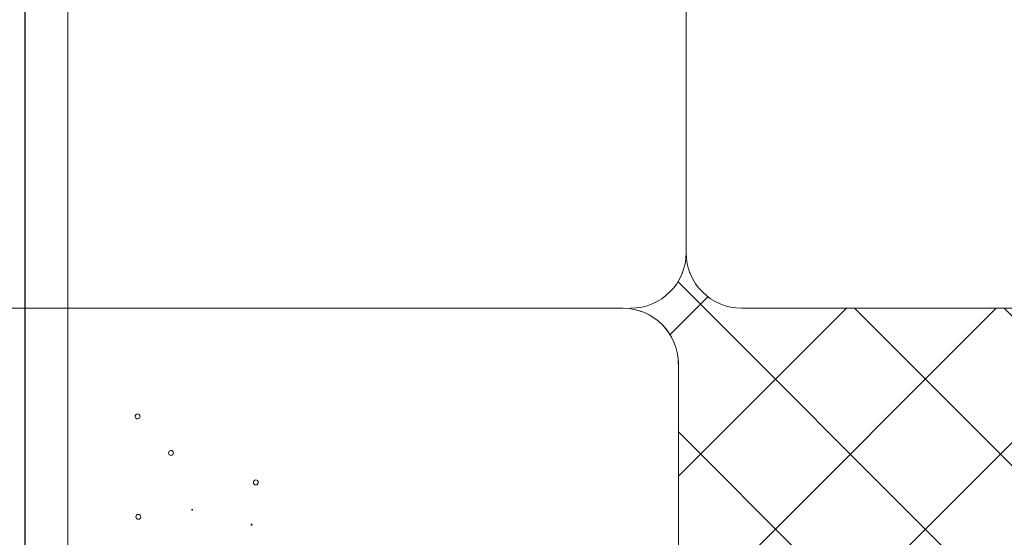
# Model space of a CAD drawing. Units: inches. Extents: x -466983 to 1020, y 324 to 318697.
# Tile 51 of 97: x 621 to 644, y 924 to 936. Entities that reach past the tile are written whole.
import ezdxf

# ---------------------------------------------------------------- set-up
doc = ezdxf.new("R2010")
doc.units = ezdxf.units.IN
doc.header["$MEASUREMENT"] = 0
doc.layers.add('A-FLOR-PATT', color=252, linetype='Continuous', lineweight=13)
doc.layers.add('A-FURN', color=8, linetype='Continuous', lineweight=18)

# ---------------------------------------------------------------- blocks, each defined once
blk = doc.blocks.new('L Shaped Sofa')
at = {"ltscale": 2}
for p, q in [((2458.96, 739.532), (2458.96, 802.773)), ((2460.8, 737.692), (2460.8, 802.773)), ((2432.683, 769.955), (2432.683, 801.818)), ((2429.959, 767.567), (2397.1, 767.567)), ((2469.187, 767.567), (2435.071, 767.567)), ((2432.347, 748.121), (2432.347, 765.179))]:
    blk.add_line(p, q, dxfattribs=at)
for centre, radius, start, end in [((2451.048, 776.875), 0.0177, 1.3946, 181.3946), ((2451.048, 776.875), 0.0177, 181.3946, 1.3946), ((2455.922, 776.541), 0.106, 1.3946, 181.3946), ((2455.922, 776.541), 0.106, 181.3946, 1.3946), ((2453.608, 776.239), 0.0177, 1.3946, 181.3946), ((2453.608, 776.239), 0.0177, 181.3946, 1.3946), ((2450.866, 775.061), 0.106, 1.3946, 181.3946), ((2450.866, 775.061), 0.106, 181.3946, 1.3946), ((2454.518, 773.793), 0.106, 1.3946, 181.3946), ((2454.518, 773.793), 0.106, 181.3946, 1.3946), ((2455.953, 772.221), 0.106, 1.3946, 181.3946), ((2455.953, 772.221), 0.106, 181.3946, 1.3946), ((2435.071, 769.955), 2.388, 180, 270), ((2429.959, 765.179), 2.388, 0, 90), ((2434.735, 765.179), 2.388, 90, 180)]:
    blk.add_arc(centre, radius, start, end, dxfattribs=at)

msp = doc.modelspace()

# ---------------------------------------------------------------- hatches: boundary and pattern name
at = {"layer": 'A-FLOR-PATT', "transparency": 33554572}
h = msp.add_hatch(dxfattribs=at)
h.set_pattern_fill('ANSI37', color=256, scale=30)
h.set_pattern_definition([(45, (-1212.4137, -290.035), (-2.6516504, 2.6516504), []), (135, (-1212.4137, -290.035), (-2.6516504, -2.6516504), [])])
h.paths.add_polyline_path([(901.806, 1075.938), (900.614, 1075.938), (900.614, 1065.386), (899.391, 1065.386), (898.091, 1065.386), (892.836, 1058.71, -0.258377), (892.188, 1058.351), (879.985, 1058.351, -0.20177), (879.438, 1058.581), (874.081, 1065.386), (872.781, 1065.386), (871.558, 1065.386), (871.558, 1075.938), (813.806, 1075.938), (813.806, 1044.792), (832.395, 1044.792, -0.394795), (848.66, 1028.536), (848.66, 1009.938), (901.806, 1009.938), (901.806, 1015.938), (901.306, 1015.938), (871.306, 1015.938), (871.306, 1017.25), (871.334, 1017.25, -0.401453), (901.306, 1045.938), (901.806, 1045.938)])
edge = h.paths.add_edge_path(flags=16)
edge.add_line((847.773, 1068.949), (847.773, 1073.709))
edge.add_arc((849.227, 1073.709), 1.454, 90, 180, ccw=False)
edge.add_line((849.227, 1075.163), (864.492, 1075.163))
edge.add_arc((864.492, 1073.709), 1.454, 0, 90, ccw=False)
edge.add_line((865.946, 1073.709), (865.946, 1069.004))
edge.add_arc((832.645, 1068.976), 33.301, -20.6123, 0.0472, ccw=False)
edge.add_ellipse((856.859, 1058.48), major_axis=(0, 10.213), ratio=0.685919, start_angle=100.0088, end_angle=259.9912, ccw=False)
edge.add_arc((881.074, 1068.976), 33.301, 180.0472, 200.6123, ccw=False)
h.paths.add_polyline_path([(853.146, 1066.482), (853.146, 1066.453), (853.146, 1066.453, 0.433107), (852.917, 1066.685), (852.917, 1066.453), (853.146, 1066.453), (853.146, 1066.482), (853.088, 1066.612, 0.697939), (852.7, 1066.453), (852.7, 1066.453), (852.7, 1066.482), (852.917, 1067.001), (852.917, 1066.685, -0.396254)], flags=0)
h.paths.add_polyline_path([(861.019, 1066.482), (861.019, 1066.453), (861.019, 1066.453, 0.416404), (860.802, 1066.685), (860.802, 1066.453), (861.019, 1066.453), (861.019, 1066.482), (860.967, 1066.605, 0.713344), (860.573, 1066.453), (860.573, 1066.453), (860.573, 1066.482), (860.802, 1067.001), (860.802, 1066.685, -0.379973)], flags=0)
edge = h.paths.add_edge_path(flags=0)
edge.add_spline(control_points=[(861.13, 1065.785), (861.466, 1065.248), (861.613, 1065.016), (861.983, 1064.374), (862.192, 1063.944), (862.561, 1063.039), (862.721, 1062.563), (862.987, 1061.578), (863.092, 1061.069), (863.245, 1060.031), (863.293, 1059.503), (863.329, 1058.441), (863.318, 1057.908), (863.237, 1056.852), (863.166, 1056.329), (862.97, 1055.308), (862.843, 1054.81), (862.537, 1053.852), (862.357, 1053.393), (861.951, 1052.525), (861.725, 1052.117), (861.233, 1051.362), (860.967, 1051.016), (860.405, 1050.395), (860.108, 1050.12), (859.494, 1049.646), (859.176, 1049.448), (858.528, 1049.13), (858.197, 1049.011), (857.531, 1048.852), (857.196, 1048.812), (856.525, 1048.812), (856.189, 1048.852), (855.524, 1049.01), (855.193, 1049.129), (854.545, 1049.447), (854.227, 1049.645), (853.612, 1050.118), (853.316, 1050.393), (852.753, 1051.014), (852.487, 1051.36), (851.995, 1052.114), (851.769, 1052.523), (851.363, 1053.39), (851.183, 1053.85), (850.877, 1054.807), (850.75, 1055.305), (850.553, 1056.326), (850.483, 1056.849), (850.401, 1057.905), (850.39, 1058.438), (850.426, 1059.5), (850.473, 1060.028), (850.626, 1061.066), (850.732, 1061.575), (850.997, 1062.561), (851.157, 1063.036), (851.525, 1063.942), (851.734, 1064.371), (852.106, 1065.016), (852.254, 1065.25), (852.608, 1065.733)], knot_values=[3.915332, 3.915332, 3.915332, 3.915332, 4.013468, 4.013468, 4.175532, 4.175532, 4.337596, 4.337596, 4.49966, 4.49966, 4.661724, 4.661724, 4.823788, 4.823788, 4.985852, 4.985852, 5.147916, 5.147916, 5.30998, 5.30998, 5.472044, 5.472044, 5.634109, 5.634109, 5.796173, 5.796173, 5.958237, 5.958237, 6.120301, 6.120301, 6.282365, 6.282365, 6.444429, 6.444429, 6.606493, 6.606493, 6.768557, 6.768557, 6.930621, 6.930621, 7.092685, 7.092685, 7.254749, 7.254749, 7.416813, 7.416813, 7.578878, 7.578878, 7.740942, 7.740942, 7.903006, 7.903006, 8.06507, 8.06507, 8.227134, 8.227134, 8.389198, 8.389198, 8.551262, 8.551262, 8.65037, 8.65037, 8.65037, 8.65037], degree=3, periodic=0)
edge.add_line((852.642, 1065.785), (861.13, 1065.785))
edge = h.paths.add_edge_path(flags=0)
edge.add_ellipse((856.85, 1057.743), major_axis=(0, 7.792), ratio=0.687861, start_angle=0, end_angle=360)
h.paths.add_polyline_path([(848.863, 1069.389), (848.863, 1073.96, -0.414214), (849.954, 1075.051), (863.765, 1075.051, -0.414214), (864.856, 1073.96), (864.856, 1069.389, -0.388936), (864.524, 1069.027, -0.043561), (849.195, 1069.027, -0.388936)], flags=0)
h.paths.add_polyline_path([(853.101, 1068.112, -1), (852.677, 1068.112, -1)], flags=0)
edge = h.paths.add_edge_path(flags=0)
edge.add_ellipse((856.859, 1057.338), major_axis=(0, 2.207), ratio=0.657164, start_angle=0, end_angle=360)
h.paths.add_polyline_path([(861.041, 1068.112, -1), (860.618, 1068.112, -1)], flags=0)
edge = h.paths.add_edge_path()
edge.add_line((573.954, 1057.341), (573.954, 1075.938))
edge.add_line((573.954, 1075.938), (558.731, 1075.938))
edge.add_line((558.731, 1075.938), (558.731, 1065.386))
edge.add_line((558.731, 1065.386), (557.507, 1065.386))
edge.add_line((557.507, 1065.386), (556.207, 1065.386))
edge.add_line((556.207, 1065.386), (550.952, 1058.71))
edge.add_arc((550.304, 1059.116), 0.765, 270, 327.9483, ccw=False)
edge.add_line((550.304, 1058.351), (538.101, 1058.351))
edge.add_arc((538.101, 1059.116), 0.765, 224.3704, 270, ccw=False)
edge.add_line((537.555, 1058.581), (532.198, 1065.386))
edge.add_line((532.198, 1065.386), (530.898, 1065.386))
edge.add_line((530.898, 1065.386), (529.674, 1065.386))
edge.add_line((529.674, 1065.386), (529.674, 1075.938))
edge.add_line((529.674, 1075.938), (520.806, 1075.938))
edge.add_line((520.806, 1075.938), (520.806, 1045.938))
edge.add_line((520.806, 1045.938), (521.306, 1045.938))
edge.add_arc((521.306, 1015.938), 30, 2.5075, 90, ccw=False)
edge.add_line((551.277, 1017.25), (551.306, 1017.25))
edge.add_line((551.306, 1017.25), (551.306, 1015.938))
edge.add_line((551.306, 1015.938), (520.806, 1015.938))
edge.add_line((520.806, 1015.938), (520.806, 1009.938))
edge.add_line((520.806, 1009.938), (559.191, 1010.402))
edge.add_arc((559.191, 1011.856), 1.454, 180, 270, ccw=False)
edge.add_line((557.737, 1011.856), (557.737, 1016.561))
edge.add_arc((591.039, 1016.589), 33.301, 159.3877, 180.0472, ccw=False)
edge.add_ellipse((566.824, 1027.085), major_axis=(0, 10.213), ratio=0.685919, start_angle=280.0088, end_angle=439.9912, ccw=False)
edge.add_arc((542.609, 1016.589), 33.301, 0.0472, 20.6123, ccw=False)
edge.add_line((575.91, 1016.616), (575.91, 1011.856))
edge.add_arc((574.456, 1011.856), 1.454, -90, 0, ccw=False)
edge.add_line((574.456, 1010.402), (608.806, 1009.938))
edge.add_line((608.806, 1009.938), (608.806, 1041.086))
edge.add_line((608.806, 1041.086), (590.218, 1041.086))
edge.add_arc((590.775, 1057.907), 16.831, 181.9277, 268.1032, ccw=False)
edge = h.paths.add_edge_path()
edge.add_ellipse((494.244, 583.62), major_axis=(0, 10.213), ratio=0.685919, start_angle=280.0088, end_angle=439.9912, ccw=False)
edge.add_arc((470.03, 573.124), 33.301, 0.0472, 20.6123, ccw=False)
edge.add_line((503.331, 573.152), (503.331, 568.392))
edge.add_arc((501.877, 568.392), 1.454, -90, 0, ccw=False)
edge.add_line((501.877, 566.938), (539.806, 566.938))
edge.add_line((539.806, 566.938), (539.806, 572.938))
edge.add_line((539.806, 572.938), (539.306, 572.938))
edge.add_line((539.306, 572.938), (509.306, 572.938))
edge.add_line((509.306, 572.938), (509.306, 574.25))
edge.add_line((509.306, 574.25), (509.334, 574.25))
edge.add_arc((539.306, 572.938), 30, 90, 177.4925, ccw=False)
edge.add_line((539.306, 602.938), (539.806, 602.938))
edge.add_line((539.806, 602.938), (539.806, 626.938))
edge.add_line((539.806, 626.938), (531.772, 626.938))
edge.add_line((531.772, 626.938), (531.772, 616.386))
edge.add_line((531.772, 616.386), (530.548, 616.386))
edge.add_line((530.548, 616.386), (529.249, 616.386))
edge.add_line((529.249, 616.386), (523.711, 609.351))
edge.add_line((523.711, 609.351), (510.777, 609.351))
edge.add_line((510.777, 609.351), (505.239, 616.386))
edge.add_line((505.239, 616.386), (503.939, 616.386))
edge.add_line((503.939, 616.386), (502.715, 616.386))
edge.add_line((502.715, 616.386), (502.715, 626.938))
edge.add_line((502.715, 626.938), (481.698, 626.938))
edge.add_line((481.698, 626.938), (481.698, 610.995))
edge.add_arc((467.27, 611.473), 14.436, 271.9277, 358.1032, ccw=False)
edge.add_line((467.756, 597.045), (451.806, 597.045))
edge.add_line((451.806, 597.045), (451.806, 584.404))
edge.add_line((451.806, 584.404), (451.806, 566.938))
edge.add_line((451.806, 566.938), (486.612, 566.938))
edge.add_arc((486.612, 568.392), 1.454, 180, 270, ccw=False)
edge.add_line((485.158, 568.392), (485.158, 573.097))
edge.add_arc((518.459, 573.124), 33.301, 159.3877, 180.0472, ccw=False)
h.paths.add_polyline_path([(836.261, 1020.733), (879.89, 1020.733), (879.89, 1039.39), (836.261, 1039.39)], flags=25)
h.paths.add_polyline_path([(549.985, 1036.749), (593.614, 1036.749), (593.614, 1055.407), (549.985, 1055.407)], flags=24)
h.paths.add_polyline_path([(475.123, 595.596), (518.752, 595.596), (518.752, 614.253), (475.123, 614.253)], flags=24)
h = msp.add_hatch(dxfattribs=at)
h.set_pattern_fill('ANSI37', color=256, scale=20)
h.set_pattern_definition([(45, (-1212.4137, -290.035), (-1.767767, 1.767767), []), (135, (-1212.4137, -290.035), (-1.767767, -1.767767), [])])
h.paths.add_polyline_path([(809.806, 870.938), (809.806, 888.152), (806.998, 888.152), (802.662, 888.152), (789.383, 888.152), (786.285, 888.152, -0.414214), (785.499, 888.937), (785.499, 900.196), (785.499, 908.47, -0.414214), (786.808, 909.779, -0.414214), (785.499, 911.088), (785.499, 929.101, -0.414214), (786.808, 930.411, -0.414214), (785.499, 931.72), (785.499, 931.904, -0.414214), (784.19, 930.595), (766.722, 930.595, -0.412359), (765.413, 931.896, -0.413741), (764.115, 930.578), (744.578, 930.422, -0.416556), (743.786, 931.207), (743.786, 933.515), (742.215, 933.515), (742.215, 952.024, -0.001344), (743.786, 952.2), (743.786, 953.938), (678.592, 953.938), (678.592, 951.131), (678.592, 946.794), (678.592, 933.515), (678.592, 930.417, -0.414214), (677.806, 929.631), (666.548, 929.631), (658.274, 929.631, -0.414214), (656.965, 930.94, -0.414214), (655.656, 929.631), (637.642, 929.631, -0.414214), (636.333, 930.94, -0.414214), (635.024, 929.631), (634.839, 929.631, -0.414214), (636.149, 928.322), (636.149, 910.854, -0.412359), (634.848, 909.545, -0.413741), (636.165, 908.247), (636.321, 888.71, -0.416556), (635.536, 887.918), (633.228, 887.918), (633.228, 886.347), (614.719, 886.347, -0.001344), (614.544, 887.918), (612.806, 887.918), (612.806, 834.938), (612.806, 752.938), (612.806, 748.938), (612.806, 697.938), (654.806, 697.938), (654.806, 701.938), (715.806, 701.938), (715.806, 737.435), (774.292, 737.435), (774.292, 795.938), (809.806, 795.938)])
h.paths.add_polyline_path([(679.276, 849.576, 0.102523), (682.148, 849.261, -0.080461), (694.543, 849.773, -0.283899), (694.482, 849.008, 0.136605), (694.407, 848.81, -0.030441), (694.543, 846.893), (694.543, 842.62), (694.543, 838.347, -0.028219), (694.425, 836.568), (694.425, 836.568, 0.196187), (694.446, 836.271, -0.302897), (694.543, 835.467, -0.080461), (682.148, 835.979, 0.102523), (679.276, 835.664, -0.58611), (678.646, 836.017), (678.646, 849.223, -0.58611)], flags=16)
h.paths.add_polyline_path([(679.517, 848.651, 0.699597), (679.476, 848.634, 1.20716), (679.194, 848.742, 0.010621)], flags=0)
h.paths.add_polyline_path([(679.492, 836.561, -0.013798), (679.918, 836.659, -0.071703), (682.853, 837.143, -0.165743), (682.166, 839.101), (682.166, 842.609), (682.166, 846.06, -0.240616), (683.473, 848.677, -0.068263), (693.929, 849.008), (693.788, 848.708), (693.788, 849.023, 0.067332), (683.473, 848.677, 0.240616), (682.166, 846.06), (682.166, 842.609), (682.166, 839.101, 0.23459), (683.461, 836.551, 0.068093), (693.788, 836.195), (693.788, 836.51), (693.93, 836.21, -0.077215), (682.242, 836.782, 0.086627), (679.528, 836.57, -0.628402), (679.503, 836.573), (679.503, 836.607, 0.910458)], flags=0)
h.paths.add_polyline_path([(679.476, 848.636), (679.207, 848.647), (679.207, 836.572, 0.913566), (679.365, 836.586), (679.476, 836.582)], flags=0)
h.paths.add_polyline_path([(679.276, 829.86, 0.102523), (682.148, 829.546, -0.080461), (694.543, 830.057, -0.283899), (694.482, 829.293, 0.136605), (694.407, 829.095, -0.030441), (694.543, 827.178), (694.543, 822.904), (694.543, 818.631, -0.028219), (694.425, 816.853), (694.425, 816.853, 0.196187), (694.446, 816.556, -0.302897), (694.543, 815.752, -0.080461), (682.148, 816.263, 0.102523), (679.276, 815.949, -0.58611), (678.646, 816.302), (678.646, 829.507, -0.58611)], flags=16)
h.paths.add_polyline_path([(679.517, 828.936, 0.699597), (679.476, 828.919, 1.20716), (679.194, 829.027, 0.010621)], flags=0)
h.paths.add_polyline_path([(679.492, 816.846, -0.013798), (679.918, 816.944, -0.071703), (682.853, 817.428, -0.165743), (682.166, 819.385), (682.166, 822.894), (682.166, 826.345, -0.240616), (683.473, 828.961, -0.068263), (693.929, 829.293), (693.788, 828.993), (693.788, 829.308, 0.067332), (683.473, 828.961, 0.240616), (682.166, 826.345), (682.166, 822.894), (682.166, 819.385, 0.23459), (683.461, 816.836, 0.068093), (693.788, 816.48), (693.788, 816.795), (693.93, 816.495, -0.077215), (682.242, 817.066, 0.086627), (679.528, 816.855, -0.628402), (679.503, 816.858), (679.503, 816.892, 0.910458)], flags=0)
h.paths.add_polyline_path([(679.476, 828.921), (679.207, 828.932), (679.207, 816.857, 0.913566), (679.365, 816.871), (679.476, 816.867)], flags=0)
h.paths.add_polyline_path([(679.276, 810.145, 0.102523), (682.148, 809.83, -0.080461), (694.543, 810.342, -0.3023), (694.447, 809.539, 0.10023), (694.406, 809.388, -0.03057), (694.543, 807.462), (694.543, 803.189), (694.543, 798.916, -0.03057), (694.406, 796.991, 0.10023), (694.447, 796.839, -0.3023), (694.543, 796.036, -0.080461), (682.148, 796.548, 0.102523), (679.276, 796.233, -0.58611), (678.646, 796.586), (678.646, 809.792, -0.58611)], flags=16)
h.paths.add_polyline_path([(679.517, 809.242, 0.699597), (679.476, 809.224, 1.20716), (679.194, 809.332, 0.010621)], flags=0)
h.paths.add_polyline_path([(679.492, 797.151, -0.013798), (679.918, 797.25, -0.071703), (682.853, 797.734, -0.165743), (682.166, 799.691), (682.166, 803.2), (682.166, 806.65, -0.239349), (683.461, 809.258, -0.072465), (694.447, 809.541, 0.197932), (694.425, 809.241), (693.788, 809.299), (693.788, 809.614, 0.068093), (683.461, 809.258, 0.239349), (682.166, 806.65), (682.166, 803.2), (682.166, 799.691, 0.235854), (683.473, 797.132, 0.067332), (693.788, 796.786), (693.788, 797.101), (694.425, 797.159, 0.197932), (694.447, 796.859, -0.080419), (682.156, 797.379, 0.083867), (679.528, 797.16, -0.628402), (679.503, 797.164), (679.503, 797.197, 0.910458)], flags=0)
h.paths.add_polyline_path([(679.207, 809.237), (679.207, 797.162, 0.913566), (679.365, 797.176), (679.476, 797.173), (679.476, 809.227)], flags=0)
h.paths.add_polyline_path([(695.364, 853.299), (728.223, 853.299), (728.223, 771.152), (695.364, 771.152)], flags=16)
h.paths.add_polyline_path([(696.021, 852.642), (727.566, 852.642), (727.566, 771.809), (696.021, 771.809)], flags=0)
h.paths.add_polyline_path([(679.276, 788.787, 0.102523), (682.148, 788.472, -0.080461), (694.543, 788.984, -0.3023), (694.447, 788.181, 0.10023), (694.406, 788.03, -0.03057), (694.543, 786.104), (694.543, 781.831), (694.543, 777.558, -0.03057), (694.406, 775.632, 0.10023), (694.447, 775.481, -0.3023), (694.543, 774.678, -0.080461), (682.148, 775.19, 0.102523), (679.276, 774.875, -0.58611), (678.646, 775.228), (678.646, 788.434, -0.58611)], flags=16)
h.paths.add_polyline_path([(679.517, 787.883, 0.699597), (679.476, 787.866, 1.20716), (679.194, 787.974, 0.010621)], flags=0)
h.paths.add_polyline_path([(679.492, 775.793, -0.013798), (679.918, 775.891, -0.071703), (682.853, 776.375, -0.165743), (682.166, 778.333), (682.166, 781.841), (682.166, 785.292, -0.239349), (683.461, 787.899, -0.072465), (694.447, 788.182, 0.197932), (694.425, 787.882), (693.788, 787.94), (693.788, 788.255, 0.068093), (683.461, 787.899, 0.239349), (682.166, 785.292), (682.166, 781.841), (682.166, 778.333, 0.235854), (683.473, 775.774, 0.067332), (693.788, 775.428), (693.788, 775.742), (694.425, 775.8, 0.197932), (694.447, 775.5, -0.080419), (682.156, 776.021, 0.083867), (679.528, 775.802, -0.628402), (679.503, 775.805), (679.503, 775.839, 0.910458)], flags=0)
h.paths.add_polyline_path([(679.207, 787.879), (679.207, 775.804, 0.913566), (679.365, 775.818), (679.476, 775.814), (679.476, 787.868)], flags=0)
h.paths.add_polyline_path([(704.641, 854.12, -0.080461), (705.153, 866.516, 0.102523), (704.838, 869.387, -0.58611), (705.191, 870.017), (718.397, 870.017, -0.58611), (718.75, 869.387, 0.102523), (718.435, 866.516, -0.080461), (718.946, 854.12, -0.3023), (718.144, 854.217, 0.10023), (717.992, 854.257, -0.03057), (716.067, 854.12), (711.794, 854.12), (707.521, 854.12, -0.03057), (705.595, 854.257, 0.10023), (705.444, 854.217, -0.3023)], flags=16)
h.paths.add_polyline_path([(717.846, 869.146, 0.699597), (717.829, 869.187, 1.20716), (717.937, 869.47, 0.010621)], flags=0)
h.paths.add_polyline_path([(705.463, 854.216, -0.080419), (705.984, 866.507, 0.083867), (705.765, 869.135, -0.628402), (705.768, 869.16), (705.802, 869.16, 0.910458), (705.756, 869.171, -0.013798), (705.854, 868.745, -0.071703), (706.338, 865.81, -0.165743), (708.295, 866.497), (711.804, 866.497), (715.255, 866.497, -0.239349), (717.862, 865.202, -0.072465), (718.145, 854.216, 0.197932), (717.845, 854.238), (717.903, 854.876), (718.218, 854.876, 0.068093), (717.862, 865.202, 0.239349), (715.255, 866.497), (711.804, 866.497), (708.295, 866.497, 0.235854), (705.737, 865.19, 0.067332), (705.391, 854.876), (705.705, 854.876), (705.763, 854.238, 0.197932)], flags=16)
h.paths.add_polyline_path([(705.766, 869.456, 0.913566), (705.781, 869.299), (705.777, 869.187), (717.831, 869.187), (717.842, 869.456)], flags=0)
h.paths.add_polyline_path([(729.045, 842.62), (729.045, 846.893, -0.03057), (729.182, 848.818, 0.10023), (729.141, 848.97, -0.3023), (729.045, 849.773, -0.080461), (741.44, 849.261, 0.102523), (744.311, 849.576, -0.58611), (744.942, 849.223), (744.942, 836.017, -0.58611), (744.311, 835.664, 0.102523), (741.44, 835.979, -0.080461), (729.045, 835.467, -0.3023), (729.141, 836.27, 0.10023), (729.182, 836.421, -0.03057), (729.045, 838.347)], flags=16)
h.paths.add_polyline_path([(744.111, 836.585, 1.20716), (744.394, 836.477, 0.010621), (744.07, 836.567, 0.699597)], flags=0)
h.paths.add_polyline_path([(729.141, 836.268, 0.197932), (729.162, 836.568), (729.8, 836.51), (729.8, 836.195, 0.068093), (740.126, 836.551, 0.239349), (741.421, 839.159), (741.421, 842.609), (741.421, 846.118, 0.235854), (740.114, 848.677, 0.067332), (729.8, 849.023), (729.8, 848.708), (729.162, 848.65, 0.197932), (729.141, 848.95, -0.080419), (741.432, 848.43, 0.083867), (744.059, 848.649, -0.628402), (744.085, 848.645), (744.085, 848.612, 0.910458), (744.095, 848.658, -0.013798), (743.67, 848.559, -0.071703), (740.734, 848.075, -0.165743), (741.421, 846.118), (741.421, 842.609), (741.421, 839.159, -0.239349), (740.126, 836.551, -0.072465)], flags=0)
h.paths.add_polyline_path([(729.045, 830.057, -0.080461), (741.44, 829.546, 0.102523), (744.311, 829.86, -0.58611), (744.942, 829.507), (744.942, 816.302, -0.58611), (744.311, 815.949, 0.102523), (741.44, 816.263, -0.080461), (729.045, 815.752, -0.3023), (729.141, 816.554, 0.10023), (729.182, 816.706, -0.03057), (729.045, 818.631), (729.045, 822.904), (729.045, 827.178, -0.03057), (729.182, 829.103, 0.10023), (729.141, 829.255, -0.3023)], flags=16)
h.paths.add_polyline_path([(744.111, 816.869, 1.20716), (744.394, 816.761, 0.010621), (744.07, 816.852, 0.699597)], flags=0)
h.paths.add_polyline_path([(729.141, 829.235, -0.080419), (741.432, 828.714, 0.083867), (744.059, 828.933, -0.628402), (744.085, 828.93), (744.085, 828.896, 0.910458), (744.095, 828.943, -0.013798), (743.67, 828.844, -0.071703), (740.734, 828.36, -0.165743), (741.421, 826.403), (741.421, 822.894), (741.421, 819.443, -0.239349), (740.126, 816.836, -0.072465), (729.141, 816.553, 0.197932), (729.162, 816.853), (729.8, 816.795), (729.8, 816.48, 0.068093), (740.126, 816.836, 0.239349), (741.421, 819.443), (741.421, 822.894), (741.421, 826.403, 0.235854), (740.114, 828.961, 0.067332), (729.8, 829.308), (729.8, 828.993), (729.162, 828.935, 0.197932)], flags=16)
h.paths.add_polyline_path([(729.045, 810.342, -0.080461), (741.44, 809.83, 0.102523), (744.311, 810.145, -0.58611), (744.942, 809.792), (744.942, 796.586, -0.58611), (744.311, 796.233, 0.102523), (741.44, 796.548, -0.080461), (729.045, 796.036, -0.283899), (729.105, 796.801, 0.136605), (729.181, 796.999, -0.030441), (729.045, 798.916), (729.045, 803.189), (729.045, 807.462, -0.028219), (729.163, 809.241), (729.162, 809.241, 0.196187), (729.142, 809.538, -0.302897)], flags=16)
h.paths.add_polyline_path([(744.111, 797.175, 1.20716), (744.394, 797.067, 0.010621), (744.07, 797.158, 0.699597)], flags=0)
h.paths.add_polyline_path([(741.345, 809.027, 0.086627), (744.059, 809.239, -0.628402), (744.085, 809.235), (744.085, 809.202, 0.910458), (744.095, 809.248, -0.013798), (743.67, 809.15, -0.071703), (740.734, 808.666, -0.165743), (741.421, 806.708), (741.421, 803.2), (741.421, 799.749, -0.240616), (740.114, 797.132, -0.068263), (729.658, 796.801), (729.8, 797.101), (729.8, 796.786, 0.067332), (740.114, 797.132, 0.240616), (741.421, 799.749), (741.421, 803.2), (741.421, 806.708, 0.23459), (740.126, 809.258, 0.068093), (729.8, 809.614), (729.8, 809.299), (729.658, 809.599, -0.077215)], flags=0)
h.paths.add_polyline_path([(704.641, 770.33, -0.283899), (705.405, 770.27, 0.136605), (705.603, 770.194, -0.030441), (707.521, 770.33), (711.794, 770.33), (716.067, 770.33, -0.028219), (717.845, 770.212), (717.845, 770.213, 0.196187), (718.143, 770.233, -0.302897), (718.946, 770.33, -0.080461), (718.435, 757.935, 0.102523), (718.75, 755.064, -0.58611), (718.397, 754.433), (705.191, 754.433, -0.58611), (704.838, 755.064, 0.102523), (705.153, 757.935, -0.080461)], flags=16)
h.paths.add_polyline_path([(705.762, 755.305, 0.699597), (705.779, 755.264, 1.20716), (705.671, 754.981, 0.010621)], flags=0)
h.paths.add_polyline_path([(705.405, 769.717), (705.705, 769.575), (705.391, 769.575, 0.067332), (705.737, 759.261, 0.240616), (708.353, 757.954), (711.804, 757.954), (715.313, 757.954, 0.23459), (717.862, 759.249, 0.068093), (718.218, 769.575), (717.903, 769.575), (718.203, 769.717, -0.077215), (717.632, 758.03, 0.086627), (717.843, 755.316, -0.628402), (717.84, 755.29), (717.806, 755.29, 0.910458), (717.853, 755.28, -0.013798), (717.754, 755.705, -0.071703), (717.27, 758.641, -0.165743), (715.313, 757.954), (711.804, 757.954), (708.353, 757.954, -0.240616), (705.737, 759.261, -0.068263)], flags=0)
h.paths.add_polyline_path([(729.045, 788.984, -0.080461), (741.44, 788.472, 0.102523), (744.311, 788.787, -0.58611), (744.942, 788.434), (744.942, 775.228, -0.58611), (744.311, 774.875, 0.102523), (741.44, 775.19, -0.080461), (729.045, 774.678, -0.283899), (729.105, 775.443, 0.136605), (729.181, 775.64, -0.030441), (729.045, 777.558), (729.045, 781.831), (729.045, 786.104, -0.028219), (729.163, 787.882), (729.162, 787.882, 0.196187), (729.142, 788.18, -0.302897)], flags=16)
h.paths.add_polyline_path([(744.111, 775.817, 1.20716), (744.394, 775.709, 0.010621), (744.07, 775.799, 0.699597)], flags=0)
h.paths.add_polyline_path([(741.345, 787.669, 0.086627), (744.059, 787.881, -0.628402), (744.085, 787.877), (744.085, 787.844, 0.910458), (744.095, 787.89, -0.013798), (743.67, 787.791, -0.071703), (740.734, 787.307, -0.165743), (741.421, 785.35), (741.421, 781.841), (741.421, 778.39, -0.240616), (740.114, 775.774, -0.068263), (729.658, 775.443), (729.8, 775.742), (729.8, 775.428, 0.067332), (740.114, 775.774, 0.240616), (741.421, 778.39), (741.421, 781.841), (741.421, 785.35, 0.23459), (740.126, 787.899, 0.068093), (729.8, 788.255), (729.8, 787.94), (729.658, 788.241, -0.077215)], flags=0)
h.paths.add_polyline_path([(744.111, 848.636), (744.111, 836.582), (744.381, 836.572), (744.381, 848.647, 0.913566), (744.223, 848.633)], flags=0)
h.paths.add_polyline_path([(744.223, 828.917), (744.111, 828.921), (744.111, 816.867), (744.381, 816.857), (744.381, 828.932, 0.913566)], flags=0)
h.paths.add_polyline_path([(717.831, 755.264), (705.777, 755.264), (705.766, 754.994), (717.842, 754.994, 0.913566), (717.827, 755.152)], flags=0)
h.paths.add_polyline_path([(744.223, 809.223), (744.111, 809.227), (744.111, 797.173), (744.381, 797.162), (744.381, 809.237, 0.913566)], flags=0)
h.paths.add_polyline_path([(744.111, 787.868), (744.111, 775.814), (744.381, 775.804), (744.381, 787.879, 0.913566), (744.223, 787.865)], flags=0)
h.paths.add_polyline_path([(678.877, 877.123), (737.613, 877.123), (737.613, 899.512), (678.877, 899.512)], flags=24)

# ---------------------------------------------------------------- linework, layer by layer
at = {"layer": 'A-FURN', "ltscale": 2}
for p, q in [((620.734, 946.009), (620.734, 910.331)), ((620.734, 946.009), (620.734, 910.331)), ((620.734, 946.009), (620.734, 910.331)), ((620.734, 946.009), (620.734, 910.331)), ((620.734, 946.009), (620.734, 910.331)), ((620.734, 946.009), (620.734, 910.331)), ((621.743, 945), (621.743, 910.331)), ((621.743, 945), (621.743, 910.331)), ((621.743, 945), (621.743, 910.331)), ((621.743, 945), (621.743, 910.331)), ((621.743, 945), (621.743, 910.331)), ((621.743, 945), (621.743, 910.331)), ((636.333, 940.292), (636.333, 930.94)), ((636.333, 940.292), (636.333, 930.94)), ((636.333, 940.292), (636.333, 930.94)), ((636.333, 940.292), (636.333, 930.94)), ((636.333, 940.292), (636.333, 930.94)), ((636.333, 940.292), (636.333, 930.94)), ((616.137, 929.631), (634.839, 929.631)), ((616.137, 929.631), (634.839, 929.631)), ((616.137, 929.631), (634.839, 929.631)), ((616.137, 929.631), (634.839, 929.631)), ((616.137, 929.631), (634.839, 929.631)), ((616.137, 929.631), (634.839, 929.631)), ((637.642, 929.631), (655.656, 929.631)), ((637.642, 929.631), (655.656, 929.631)), ((637.642, 929.631), (655.656, 929.631)), ((637.642, 929.631), (655.656, 929.631)), ((637.642, 929.631), (655.656, 929.631)), ((637.642, 929.631), (655.656, 929.631)), ((636.149, 928.322), (636.149, 910.854)), ((636.149, 928.322), (636.149, 910.854)), ((636.149, 928.322), (636.149, 910.854)), ((636.149, 928.322), (636.149, 910.854)), ((636.149, 928.322), (636.149, 910.854)), ((636.149, 928.322), (636.149, 910.854))]:
    msp.add_line(p, q, dxfattribs=at)
for centre, radius, start, end in [((635.024, 930.94), 1.309, 270, 0), ((635.024, 930.94), 1.309, 270, 0), ((635.024, 930.94), 1.309, 270, 0), ((635.024, 930.94), 1.309, 270, 0), ((635.024, 930.94), 1.309, 270, 0), ((635.024, 930.94), 1.309, 270, 0), ((637.642, 930.94), 1.309, 180, 270), ((637.642, 930.94), 1.309, 180, 270), ((637.642, 930.94), 1.309, 180, 270), ((637.642, 930.94), 1.309, 180, 270), ((637.642, 930.94), 1.309, 180, 270), ((637.642, 930.94), 1.309, 180, 270), ((634.839, 928.322), 1.309, 0, 90), ((634.839, 928.322), 1.309, 0, 90), ((634.839, 928.322), 1.309, 0, 90), ((634.839, 928.322), 1.309, 0, 90), ((634.839, 928.322), 1.309, 0, 90), ((634.839, 928.322), 1.309, 0, 90), ((623.391, 927.08), 0.0582, 1.3946, 181.3946), ((623.391, 927.08), 0.0582, 1.3946, 181.3946), ((623.391, 927.08), 0.0582, 1.3946, 181.3946), ((623.391, 927.08), 0.0582, 1.3946, 181.3946), ((623.391, 927.08), 0.0582, 1.3946, 181.3946), ((623.391, 927.08), 0.0582, 1.3946, 181.3946), ((623.391, 927.08), 0.0582, 181.3946, 1.3946), ((623.391, 927.08), 0.0582, 181.3946, 1.3946), ((623.391, 927.08), 0.0582, 181.3946, 1.3946), ((623.391, 927.08), 0.0582, 181.3946, 1.3946), ((623.391, 927.08), 0.0582, 181.3946, 1.3946), ((623.391, 927.08), 0.0582, 181.3946, 1.3946), ((624.178, 926.218), 0.0582, 1.3946, 181.3946), ((624.178, 926.218), 0.0582, 1.3946, 181.3946), ((624.178, 926.218), 0.0582, 1.3946, 181.3946), ((624.178, 926.218), 0.0582, 1.3946, 181.3946), ((624.178, 926.218), 0.0582, 1.3946, 181.3946), ((624.178, 926.218), 0.0582, 1.3946, 181.3946), ((624.178, 926.218), 0.0582, 181.3946, 1.3946), ((624.178, 926.218), 0.0582, 181.3946, 1.3946), ((624.178, 926.218), 0.0582, 181.3946, 1.3946), ((624.178, 926.218), 0.0582, 181.3946, 1.3946), ((624.178, 926.218), 0.0582, 181.3946, 1.3946), ((624.178, 926.218), 0.0582, 181.3946, 1.3946), ((626.181, 925.523), 0.0582, 1.3946, 181.3946), ((626.181, 925.523), 0.0582, 1.3946, 181.3946), ((626.181, 925.523), 0.0582, 1.3946, 181.3946), ((626.181, 925.523), 0.0582, 1.3946, 181.3946), ((626.181, 925.523), 0.0582, 1.3946, 181.3946), ((626.181, 925.523), 0.0582, 1.3946, 181.3946), ((626.181, 925.523), 0.0582, 181.3946, 1.3946), ((626.181, 925.523), 0.0582, 181.3946, 1.3946), ((626.181, 925.523), 0.0582, 181.3946, 1.3946), ((626.181, 925.523), 0.0582, 181.3946, 1.3946), ((626.181, 925.523), 0.0582, 181.3946, 1.3946), ((626.181, 925.523), 0.0582, 181.3946, 1.3946), ((624.677, 924.877), 0.0097, 1.3946, 181.3946), ((624.677, 924.877), 0.0097, 1.3946, 181.3946), ((624.677, 924.877), 0.0097, 1.3946, 181.3946), ((624.677, 924.877), 0.0097, 1.3946, 181.3946), ((624.677, 924.877), 0.0097, 1.3946, 181.3946), ((624.677, 924.877), 0.0097, 1.3946, 181.3946), ((624.677, 924.877), 0.0097, 181.3946, 1.3946), ((624.677, 924.877), 0.0097, 181.3946, 1.3946), ((624.677, 924.877), 0.0097, 181.3946, 1.3946), ((624.677, 924.877), 0.0097, 181.3946, 1.3946), ((624.677, 924.877), 0.0097, 181.3946, 1.3946), ((624.677, 924.877), 0.0097, 181.3946, 1.3946), ((623.408, 924.711), 0.0582, 1.3946, 181.3946), ((623.408, 924.711), 0.0582, 1.3946, 181.3946), ((623.408, 924.711), 0.0582, 1.3946, 181.3946), ((623.408, 924.711), 0.0582, 1.3946, 181.3946), ((623.408, 924.711), 0.0582, 1.3946, 181.3946), ((623.408, 924.711), 0.0582, 1.3946, 181.3946), ((623.408, 924.711), 0.0582, 181.3946, 1.3946), ((623.408, 924.711), 0.0582, 181.3946, 1.3946), ((623.408, 924.711), 0.0582, 181.3946, 1.3946), ((623.408, 924.711), 0.0582, 181.3946, 1.3946), ((623.408, 924.711), 0.0582, 181.3946, 1.3946), ((623.408, 924.711), 0.0582, 181.3946, 1.3946), ((626.081, 924.528), 0.0097, 1.3946, 181.3946), ((626.081, 924.528), 0.0097, 1.3946, 181.3946), ((626.081, 924.528), 0.0097, 1.3946, 181.3946), ((626.081, 924.528), 0.0097, 1.3946, 181.3946), ((626.081, 924.528), 0.0097, 1.3946, 181.3946), ((626.081, 924.528), 0.0097, 1.3946, 181.3946), ((626.081, 924.528), 0.0097, 181.3946, 1.3946), ((626.081, 924.528), 0.0097, 181.3946, 1.3946), ((626.081, 924.528), 0.0097, 181.3946, 1.3946), ((626.081, 924.528), 0.0097, 181.3946, 1.3946), ((626.081, 924.528), 0.0097, 181.3946, 1.3946), ((626.081, 924.528), 0.0097, 181.3946, 1.3946)]:
    msp.add_arc(centre, radius, start, end, dxfattribs=at)

# ---------------------------------------------------------------- block references
at = {"layer": 'A-FURN', "xscale": 0.5482153745360612, "yscale": 0.5482153745360612, "zscale": 0.5482153745360612, "rotation": 180}
msp.add_blockref('L Shaped Sofa', (1969.783, 1350.423), dxfattribs=at)

doc.saveas('drawing.dxf')
